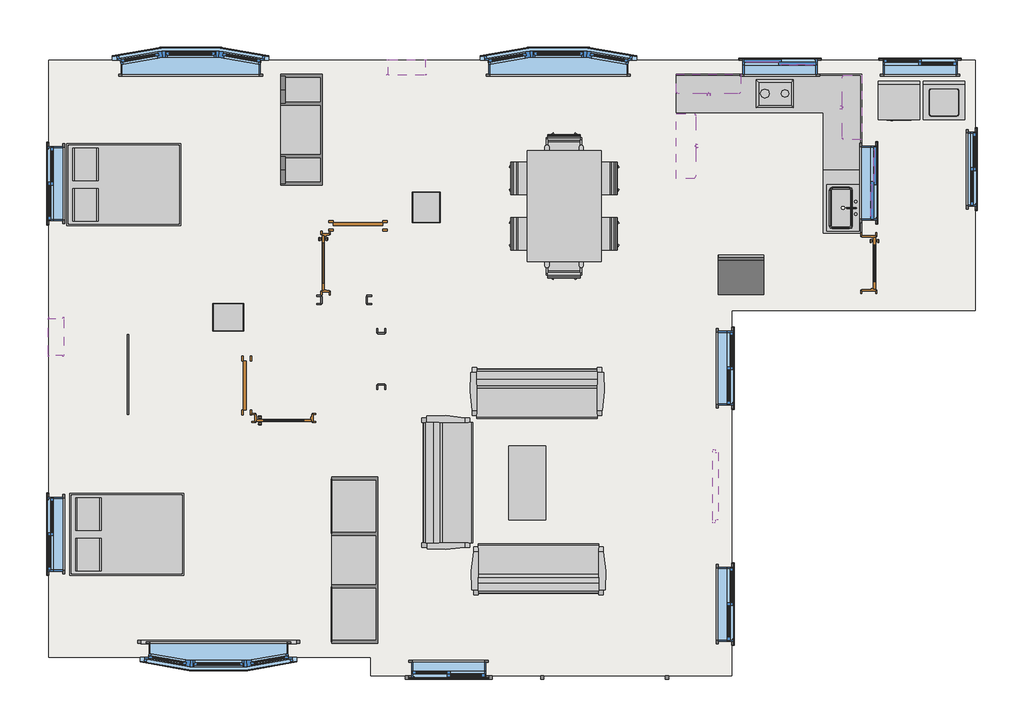
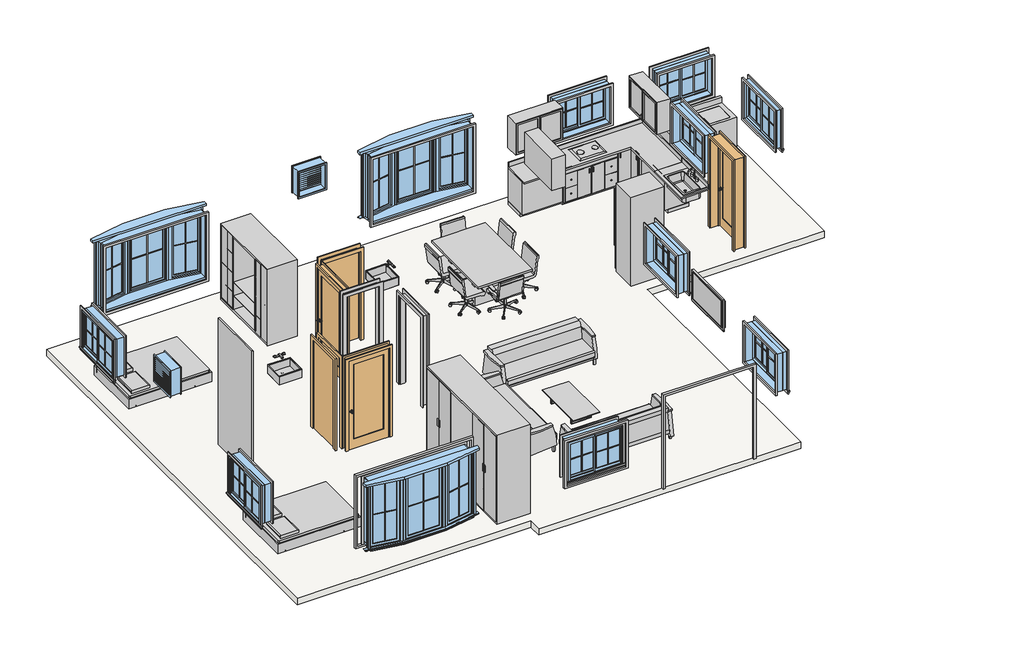
# One storey, incomplete: 54 proxies, 27 furniture elements, 14 windows, 5 doors, 3 flow terminals, 1 plate, 1 slab.
"""IFC4 building model written with IfcOpenShell, lengths in millimetres."""

from ifc_helpers import new_model, si_unit, frame, origin, place, context, project, spatial, polyline, outline, extrude, transform, mapped, element, save
from components import proxy_3c1fa1d0, proxy_97c73763, muntin_pattern_2x2_muntin_pattern_2x2_d8607f27, muntin_pattern_2x2_muntin_pattern_2x2_395d1e8c, muntin_pattern_2x2_muntin_pattern_2x2_0ac132d2, proxy_7d9a186d, proxy_dc468f74, proxy_76352e5b, trim_window_exterior_flat_with_sill_c4e67c73, trim_window_interior_flat_picture_frame_9ca7b173, trim_window_interior_flat_picture_frame_cf1733af, proxy_e75280ca, door_e2f2f551, door_a3feeac7, door_38851409, flow_terminal_cce4e9d2, flow_terminal_4d548711, furniture_e236c193, furniture_f415afdb, furniture_13b99e4d, furniture_b58f7881, casework_2_casework_2_327cef27, casework_3_casework_3_ac713c45, chair_task_chair_task_b7f3823b, chair_task_arms_chair_task_arms_fa5a08ef, furniture_738e865d, furniture_f6f93809, furniture_88072bd9, furniture_1f19b6cd, furniture_4a9d42a7, furniture_0c59c13b, furniture_0bcc43ae, furniture_5e39d705, furniture_92d3ea51, furniture_19fd8281, system_panel_glazed_349e9711, window_bf21e6cb, window_f2d8fef0, window_2eef0573, window_a4a981b4

model = new_model("IFC4")

# Units and contexts
model_context = context("Model", 3, world=origin())
ifc_project = project(units=[si_unit("LENGTHUNIT", "METRE", prefix="MILLI")], contexts=[model_context])

# Site, building, storey
site = spatial("IfcSite", under=ifc_project)
building = spatial("IfcBuilding", under=site)
storey = spatial("IfcBuildingStorey", under=building, Elevation=609.6)

# Proxies
placement = place(None, origin())
proxy_shape = proxy_3c1fa1d0(model_context)
element("IfcBuildingElementProxy", 1, Name="Cook Top-2 Unit : 12\" x 18\" 2", ObjectType="Cook Top-2 Unit : 12\" x 18\" 2", at=placement, inside=storey, context=model_context, shape_type="MappedRepresentation", body=[
    mapped(proxy_shape, transform((-6059.4169457, 11972.2965218, 609.6), x_axis=(0.0, 1.0, 0.0), y_axis=(-1.0, 0.0, 0.0), z_axis=(0.0, 0.0, 1.0))),
])
proxy_2_shape = proxy_97c73763(model_context)
element("IfcBuildingElementProxy", 2, Name="Dryer : 27\" x 25\" x 35\"", ObjectType="Dryer : 27\" x 25\" x 35\"", at=placement, inside=storey, context=model_context, shape_type="MappedRepresentation", body=[
    mapped(proxy_2_shape, transform((-4423.9291976, 11619.535518, 609.6), x_axis=(1.0, 0.0, 0.0), y_axis=(0.0, 1.0, 0.0), z_axis=(0.0, 0.0, 1.0))),
])
muntin_pattern_2x2_muntin_pattern_2x2_shape = muntin_pattern_2x2_muntin_pattern_2x2_d8607f27(model_context)
element("IfcBuildingElementProxy", 3, Name="Muntin Pattern_2x2 : Muntin Pattern_2x2", ObjectType="Muntin Pattern_2x2 : Muntin Pattern_2x2", at=placement, inside=storey, context=model_context, shape_type="MappedRepresentation", body=[
    mapped(muntin_pattern_2x2_muntin_pattern_2x2_shape, transform((-15243.1667413, 2653.6715218, 1339.85), x_axis=(-1.0, 0.0, 0.0), y_axis=(0.0, -1.0, 0.0), z_axis=(0.0, 0.0, 1.0))),
])
element("IfcBuildingElementProxy", 4, Name="Muntin Pattern_2x2 : Muntin Pattern_2x2", ObjectType="Muntin Pattern_2x2 : Muntin Pattern_2x2", at=placement, inside=storey, context=model_context, shape_type="MappedRepresentation", body=[
    mapped(muntin_pattern_2x2_muntin_pattern_2x2_shape, transform((-15700.3667413, 12705.7215218, 1339.85), x_axis=(1.0, 0.0, 0.0), y_axis=(0.0, 1.0, 0.0), z_axis=(0.0, 0.0, 1.0))),
])
element("IfcBuildingElementProxy", 5, Name="Muntin Pattern_2x2 : Muntin Pattern_2x2", ObjectType="Muntin Pattern_2x2 : Muntin Pattern_2x2", at=placement, inside=storey, context=model_context, shape_type="MappedRepresentation", body=[
    mapped(muntin_pattern_2x2_muntin_pattern_2x2_shape, transform((-9651.9917413, 12705.7215218, 1339.85), x_axis=(1.0, 0.0, 0.0), y_axis=(0.0, 1.0, 0.0), z_axis=(0.0, 0.0, 1.0))),
])
muntin_pattern_2x2_muntin_pattern_2x2_2_shape = muntin_pattern_2x2_muntin_pattern_2x2_395d1e8c(model_context)
element("IfcBuildingElementProxy", 6, Name="Muntin Pattern_2x2 : Muntin Pattern_2x2", ObjectType="Muntin Pattern_2x2 : Muntin Pattern_2x2", at=placement, inside=storey, context=model_context, shape_type="MappedRepresentation", body=[
    mapped(muntin_pattern_2x2_muntin_pattern_2x2_2_shape, transform((-14406.7973738, 2718.2624794, 1339.85), x_axis=(-0.9848077530122097, -0.17364817766692092, 0.0), y_axis=(0.17364817766692092, -0.9848077530122097, 0.0), z_axis=(0.0, 0.0, 1.0))),
])
element("IfcBuildingElementProxy", 7, Name="Muntin Pattern_2x2 : Muntin Pattern_2x2", ObjectType="Muntin Pattern_2x2 : Muntin Pattern_2x2", at=placement, inside=storey, context=model_context, shape_type="MappedRepresentation", body=[
    mapped(muntin_pattern_2x2_muntin_pattern_2x2_2_shape, transform((-16079.5361088, 2718.2624794, 1339.85), x_axis=(-0.9848077530122065, 0.17364817766693974, 0.0), y_axis=(-0.17364817766693974, -0.9848077530122065, 0.0), z_axis=(0.0, 0.0, 1.0))),
])
element("IfcBuildingElementProxy", 8, Name="Muntin Pattern_2x2 : Muntin Pattern_2x2", ObjectType="Muntin Pattern_2x2 : Muntin Pattern_2x2", at=placement, inside=storey, context=model_context, shape_type="MappedRepresentation", body=[
    mapped(muntin_pattern_2x2_muntin_pattern_2x2_2_shape, transform((-16536.7361088, 12641.1305642, 1339.85), x_axis=(0.9848077530122097, 0.17364817766692092, 0.0), y_axis=(-0.17364817766692092, 0.9848077530122097, 0.0), z_axis=(0.0, 0.0, 1.0))),
])
element("IfcBuildingElementProxy", 9, Name="Muntin Pattern_2x2 : Muntin Pattern_2x2", ObjectType="Muntin Pattern_2x2 : Muntin Pattern_2x2", at=placement, inside=storey, context=model_context, shape_type="MappedRepresentation", body=[
    mapped(muntin_pattern_2x2_muntin_pattern_2x2_2_shape, transform((-14863.9973738, 12641.1305642, 1339.85), x_axis=(0.9848077530122065, -0.17364817766693974, 0.0), y_axis=(0.17364817766693974, 0.9848077530122065, 0.0), z_axis=(0.0, 0.0, 1.0))),
])
element("IfcBuildingElementProxy", 10, Name="Muntin Pattern_2x2 : Muntin Pattern_2x2", ObjectType="Muntin Pattern_2x2 : Muntin Pattern_2x2", at=placement, inside=storey, context=model_context, shape_type="MappedRepresentation", body=[
    mapped(muntin_pattern_2x2_muntin_pattern_2x2_2_shape, transform((-10488.3611088, 12641.1305642, 1339.85), x_axis=(0.9848077530122097, 0.17364817766692092, 0.0), y_axis=(-0.17364817766692092, 0.9848077530122097, 0.0), z_axis=(0.0, 0.0, 1.0))),
])
element("IfcBuildingElementProxy", 11, Name="Muntin Pattern_2x2 : Muntin Pattern_2x2", ObjectType="Muntin Pattern_2x2 : Muntin Pattern_2x2", at=placement, inside=storey, context=model_context, shape_type="MappedRepresentation", body=[
    mapped(muntin_pattern_2x2_muntin_pattern_2x2_2_shape, transform((-8815.6223738, 12641.1305642, 1339.85), x_axis=(0.9848077530122065, -0.17364817766693974, 0.0), y_axis=(0.17364817766693974, 0.9848077530122065, 0.0), z_axis=(0.0, 0.0, 1.0))),
])
muntin_pattern_2x2_muntin_pattern_2x2_3_shape = muntin_pattern_2x2_muntin_pattern_2x2_0ac132d2(model_context)
element("IfcBuildingElementProxy", 12, Name="Muntin Pattern_2x2 : Muntin Pattern_2x2", ObjectType="Muntin Pattern_2x2 : Muntin Pattern_2x2", at=placement, inside=storey, context=model_context, shape_type="MappedRepresentation", body=[
    mapped(muntin_pattern_2x2_muntin_pattern_2x2_3_shape, transform((-5719.7542413, 12540.6215218, 1835.15), x_axis=(1.0, 0.0, 0.0), y_axis=(0.0, 1.0, 0.0), z_axis=(0.0, 0.0, 1.0))),
])
element("IfcBuildingElementProxy", 13, Name="Muntin Pattern_2x2 : Muntin Pattern_2x2", ObjectType="Muntin Pattern_2x2 : Muntin Pattern_2x2", at=placement, inside=storey, context=model_context, shape_type="MappedRepresentation", body=[
    mapped(muntin_pattern_2x2_muntin_pattern_2x2_3_shape, transform((-6288.0792413, 12585.0715218, 1835.15), x_axis=(1.0, 0.0, 0.0), y_axis=(0.0, 1.0, 0.0), z_axis=(0.0, 0.0, 1.0))),
])
element("IfcBuildingElementProxy", 14, Name="Muntin Pattern_2x2 : Muntin Pattern_2x2", ObjectType="Muntin Pattern_2x2 : Muntin Pattern_2x2", at=placement, inside=storey, context=model_context, shape_type="MappedRepresentation", body=[
    mapped(muntin_pattern_2x2_muntin_pattern_2x2_3_shape, transform((-4486.2667413, 10291.1340218, 1809.75), x_axis=(0.0, -1.0, 0.0), y_axis=(1.0, 0.0, 0.0), z_axis=(0.0, 0.0, 1.0))),
])
element("IfcBuildingElementProxy", 15, Name="Muntin Pattern_2x2 : Muntin Pattern_2x2", ObjectType="Muntin Pattern_2x2 : Muntin Pattern_2x2", at=placement, inside=storey, context=model_context, shape_type="MappedRepresentation", body=[
    mapped(muntin_pattern_2x2_muntin_pattern_2x2_3_shape, transform((-4441.8167413, 10859.4590218, 1809.75), x_axis=(0.0, -1.0, 0.0), y_axis=(1.0, 0.0, 0.0), z_axis=(0.0, 0.0, 1.0))),
])
element("IfcBuildingElementProxy", 16, Name="Muntin Pattern_2x2 : Muntin Pattern_2x2", ObjectType="Muntin Pattern_2x2 : Muntin Pattern_2x2", at=placement, inside=storey, context=model_context, shape_type="MappedRepresentation", body=[
    mapped(muntin_pattern_2x2_muntin_pattern_2x2_3_shape, transform((-6848.4667413, 7243.1340218, 1606.55), x_axis=(0.0, -1.0, 0.0), y_axis=(1.0, 0.0, 0.0), z_axis=(0.0, 0.0, 1.0))),
])
element("IfcBuildingElementProxy", 17, Name="Muntin Pattern_2x2 : Muntin Pattern_2x2", ObjectType="Muntin Pattern_2x2 : Muntin Pattern_2x2", at=placement, inside=storey, context=model_context, shape_type="MappedRepresentation", body=[
    mapped(muntin_pattern_2x2_muntin_pattern_2x2_3_shape, transform((-6804.0167413, 7811.4590218, 1606.55), x_axis=(0.0, -1.0, 0.0), y_axis=(1.0, 0.0, 0.0), z_axis=(0.0, 0.0, 1.0))),
])
element("IfcBuildingElementProxy", 18, Name="Muntin Pattern_2x2 : Muntin Pattern_2x2", ObjectType="Muntin Pattern_2x2 : Muntin Pattern_2x2", at=placement, inside=storey, context=model_context, shape_type="MappedRepresentation", body=[
    mapped(muntin_pattern_2x2_muntin_pattern_2x2_3_shape, transform((-6848.4667413, 3356.9340218, 1606.55), x_axis=(0.0, -1.0, 0.0), y_axis=(1.0, 0.0, 0.0), z_axis=(0.0, 0.0, 1.0))),
])
element("IfcBuildingElementProxy", 19, Name="Muntin Pattern_2x2 : Muntin Pattern_2x2", ObjectType="Muntin Pattern_2x2 : Muntin Pattern_2x2", at=placement, inside=storey, context=model_context, shape_type="MappedRepresentation", body=[
    mapped(muntin_pattern_2x2_muntin_pattern_2x2_3_shape, transform((-6804.0167413, 3925.2590218, 1606.55), x_axis=(0.0, -1.0, 0.0), y_axis=(1.0, 0.0, 0.0), z_axis=(0.0, 0.0, 1.0))),
])
element("IfcBuildingElementProxy", 20, Name="Muntin Pattern_2x2 : Muntin Pattern_2x2", ObjectType="Muntin Pattern_2x2 : Muntin Pattern_2x2", at=placement, inside=storey, context=model_context, shape_type="MappedRepresentation", body=[
    mapped(muntin_pattern_2x2_muntin_pattern_2x2_3_shape, transform((-11739.5542413, 2513.9715218, 1606.55), x_axis=(-1.0, 0.0, 0.0), y_axis=(0.0, -1.0, 0.0), z_axis=(0.0, 0.0, 1.0))),
])
element("IfcBuildingElementProxy", 21, Name="Muntin Pattern_2x2 : Muntin Pattern_2x2", ObjectType="Muntin Pattern_2x2 : Muntin Pattern_2x2", at=placement, inside=storey, context=model_context, shape_type="MappedRepresentation", body=[
    mapped(muntin_pattern_2x2_muntin_pattern_2x2_3_shape, transform((-11171.2292413, 2469.5215218, 1606.55), x_axis=(-1.0, 0.0, 0.0), y_axis=(0.0, -1.0, 0.0), z_axis=(0.0, 0.0, 1.0))),
])
element("IfcBuildingElementProxy", 22, Name="Muntin Pattern_2x2 : Muntin Pattern_2x2", ObjectType="Muntin Pattern_2x2 : Muntin Pattern_2x2", at=placement, inside=storey, context=model_context, shape_type="MappedRepresentation", body=[
    mapped(muntin_pattern_2x2_muntin_pattern_2x2_3_shape, transform((-17980.0167413, 5077.7840218, 1606.55), x_axis=(0.0, 1.0, 0.0), y_axis=(-1.0, 0.0, 0.0), z_axis=(0.0, 0.0, 1.0))),
])
element("IfcBuildingElementProxy", 23, Name="Muntin Pattern_2x2 : Muntin Pattern_2x2", ObjectType="Muntin Pattern_2x2 : Muntin Pattern_2x2", at=placement, inside=storey, context=model_context, shape_type="MappedRepresentation", body=[
    mapped(muntin_pattern_2x2_muntin_pattern_2x2_3_shape, transform((-18024.4667413, 4509.4590218, 1606.55), x_axis=(0.0, 1.0, 0.0), y_axis=(-1.0, 0.0, 0.0), z_axis=(0.0, 0.0, 1.0))),
])
element("IfcBuildingElementProxy", 24, Name="Muntin Pattern_2x2 : Muntin Pattern_2x2", ObjectType="Muntin Pattern_2x2 : Muntin Pattern_2x2", at=placement, inside=storey, context=model_context, shape_type="MappedRepresentation", body=[
    mapped(muntin_pattern_2x2_muntin_pattern_2x2_3_shape, transform((-17980.0167413, 10849.9340218, 1606.55), x_axis=(0.0, 1.0, 0.0), y_axis=(-1.0, 0.0, 0.0), z_axis=(0.0, 0.0, 1.0))),
])
element("IfcBuildingElementProxy", 25, Name="Muntin Pattern_2x2 : Muntin Pattern_2x2", ObjectType="Muntin Pattern_2x2 : Muntin Pattern_2x2", at=placement, inside=storey, context=model_context, shape_type="MappedRepresentation", body=[
    mapped(muntin_pattern_2x2_muntin_pattern_2x2_3_shape, transform((-18024.4667413, 10281.6090218, 1606.55), x_axis=(0.0, 1.0, 0.0), y_axis=(-1.0, 0.0, 0.0), z_axis=(0.0, 0.0, 1.0))),
])
element("IfcBuildingElementProxy", 26, Name="Muntin Pattern_2x2 : Muntin Pattern_2x2", ObjectType="Muntin Pattern_2x2 : Muntin Pattern_2x2", at=placement, inside=storey, context=model_context, shape_type="MappedRepresentation", body=[
    mapped(muntin_pattern_2x2_muntin_pattern_2x2_3_shape, transform((-2847.9667413, 10519.7340218, 1657.35), x_axis=(0.0, -1.0, 0.0), y_axis=(1.0, 0.0, 0.0), z_axis=(0.0, 0.0, 1.0))),
])
element("IfcBuildingElementProxy", 27, Name="Muntin Pattern_2x2 : Muntin Pattern_2x2", ObjectType="Muntin Pattern_2x2 : Muntin Pattern_2x2", at=placement, inside=storey, context=model_context, shape_type="MappedRepresentation", body=[
    mapped(muntin_pattern_2x2_muntin_pattern_2x2_3_shape, transform((-2803.5167413, 11088.0590218, 1657.35), x_axis=(0.0, -1.0, 0.0), y_axis=(1.0, 0.0, 0.0), z_axis=(0.0, 0.0, 1.0))),
])
element("IfcBuildingElementProxy", 28, Name="Muntin Pattern_2x2 : Muntin Pattern_2x2", ObjectType="Muntin Pattern_2x2 : Muntin Pattern_2x2", at=placement, inside=storey, context=model_context, shape_type="MappedRepresentation", body=[
    mapped(muntin_pattern_2x2_muntin_pattern_2x2_3_shape, transform((-3414.7042413, 12540.6215218, 1708.15), x_axis=(1.0, 0.0, 0.0), y_axis=(0.0, 1.0, 0.0), z_axis=(0.0, 0.0, 1.0))),
])
element("IfcBuildingElementProxy", 29, Name="Muntin Pattern_2x2 : Muntin Pattern_2x2", ObjectType="Muntin Pattern_2x2 : Muntin Pattern_2x2", at=placement, inside=storey, context=model_context, shape_type="MappedRepresentation", body=[
    mapped(muntin_pattern_2x2_muntin_pattern_2x2_3_shape, transform((-3983.0292413, 12585.0715218, 1708.15), x_axis=(1.0, 0.0, 0.0), y_axis=(0.0, 1.0, 0.0), z_axis=(0.0, 0.0, 1.0))),
])
proxy_3_shape = proxy_7d9a186d(model_context)
element("IfcBuildingElementProxy", 30, Name="Passage Opening-Cased : 30\" x 84\"", ObjectType="Passage Opening-Cased : 30\" x 84\"", at=placement, inside=storey, context=model_context, shape_type="MappedRepresentation", body=[
    mapped(proxy_3_shape, transform((-13184.430398, 8651.2465218, 609.6), x_axis=(-1.0, 0.0, 0.0), y_axis=(0.0, -1.0, 0.0), z_axis=(0.0, 0.0, 1.0))),
])
proxy_4_shape = proxy_dc468f74(model_context)
element("IfcBuildingElementProxy", 31, Name="Passage Opening-Cased : 34\" x 84\"", ObjectType="Passage Opening-Cased : 34\" x 84\"", at=placement, inside=storey, context=model_context, shape_type="MappedRepresentation", body=[
    mapped(proxy_4_shape, transform((-12566.6417413, 7687.8851785, 609.6), x_axis=(0.0, 1.0, 0.0), y_axis=(-1.0, 0.0, 0.0), z_axis=(0.0, 0.0, 1.0))),
])
proxy_5_shape = proxy_76352e5b(model_context)
element("IfcBuildingElementProxy", 32, Name="Refrigerator-Built-in : 30\" x 24\" LH", ObjectType="Refrigerator-Built-in : 30\" x 24\" LH", at=placement, inside=storey, context=model_context, shape_type="MappedRepresentation", body=[
    mapped(proxy_5_shape, transform((-6648.4417413, 9027.8725503, 609.6), x_axis=(1.0, 0.0, 0.0), y_axis=(0.0, 1.0, 0.0), z_axis=(0.0, 0.0, 1.0))),
])
trim_window_exterior_flat_with_sill_shape = trim_window_exterior_flat_with_sill_c4e67c73(model_context)
element("IfcBuildingElementProxy", 33, Name="Trim-Window-Exterior-Flat : with Sill", ObjectType="Trim-Window-Exterior-Flat : with Sill", at=placement, inside=storey, context=model_context, shape_type="MappedRepresentation", body=[
    mapped(trim_window_exterior_flat_with_sill_shape, transform((-6003.9167413, 12594.5965218, 2667.0), x_axis=(-1.0, 0.0, 0.0), y_axis=(0.0, 0.0, 1.0), z_axis=(0.0, 1.0, 0.0))),
])
element("IfcBuildingElementProxy", 34, Name="Trim-Window-Exterior-Flat : with Sill", ObjectType="Trim-Window-Exterior-Flat : with Sill", at=placement, inside=storey, context=model_context, shape_type="MappedRepresentation", body=[
    mapped(trim_window_exterior_flat_with_sill_shape, transform((-4432.2917413, 10575.2965218, 2641.6), x_axis=(0.0, 1.0, 0.0), y_axis=(0.0, 0.0, 1.0), z_axis=(1.0, 0.0, 0.0))),
])
element("IfcBuildingElementProxy", 35, Name="Trim-Window-Exterior-Flat : with Sill", ObjectType="Trim-Window-Exterior-Flat : with Sill", at=placement, inside=storey, context=model_context, shape_type="MappedRepresentation", body=[
    mapped(trim_window_exterior_flat_with_sill_shape, transform((-6794.4917413, 7527.2965218, 2438.4), x_axis=(0.0, 1.0, 0.0), y_axis=(0.0, 0.0, 1.0), z_axis=(1.0, 0.0, 0.0))),
])
element("IfcBuildingElementProxy", 36, Name="Trim-Window-Exterior-Flat : with Sill", ObjectType="Trim-Window-Exterior-Flat : with Sill", at=placement, inside=storey, context=model_context, shape_type="MappedRepresentation", body=[
    mapped(trim_window_exterior_flat_with_sill_shape, transform((-6794.4917413, 3641.0965218, 2438.4), x_axis=(0.0, 1.0, 0.0), y_axis=(0.0, 0.0, 1.0), z_axis=(1.0, 0.0, 0.0))),
])
element("IfcBuildingElementProxy", 37, Name="Trim-Window-Exterior-Flat : with Sill", ObjectType="Trim-Window-Exterior-Flat : with Sill", at=placement, inside=storey, context=model_context, shape_type="MappedRepresentation", body=[
    mapped(trim_window_exterior_flat_with_sill_shape, transform((-11455.3917413, 2459.9965218, 2438.4), x_axis=(1.0, 0.0, 0.0), y_axis=(0.0, 0.0, 1.0), z_axis=(0.0, -1.0, 0.0))),
])
element("IfcBuildingElementProxy", 38, Name="Trim-Window-Exterior-Flat : with Sill", ObjectType="Trim-Window-Exterior-Flat : with Sill", at=placement, inside=storey, context=model_context, shape_type="MappedRepresentation", body=[
    mapped(trim_window_exterior_flat_with_sill_shape, transform((-18033.9917413, 4793.6215218, 2438.4), x_axis=(0.0, -1.0, 0.0), y_axis=(0.0, 0.0, 1.0), z_axis=(-1.0, 0.0, 0.0))),
])
element("IfcBuildingElementProxy", 39, Name="Trim-Window-Exterior-Flat : with Sill", ObjectType="Trim-Window-Exterior-Flat : with Sill", at=placement, inside=storey, context=model_context, shape_type="MappedRepresentation", body=[
    mapped(trim_window_exterior_flat_with_sill_shape, transform((-18033.9917413, 10565.7715218, 2438.4), x_axis=(0.0, -1.0, 0.0), y_axis=(0.0, 0.0, 1.0), z_axis=(-1.0, 0.0, 0.0))),
])
element("IfcBuildingElementProxy", 40, Name="Trim-Window-Exterior-Flat : with Sill", ObjectType="Trim-Window-Exterior-Flat : with Sill", at=placement, inside=storey, context=model_context, shape_type="MappedRepresentation", body=[
    mapped(trim_window_exterior_flat_with_sill_shape, transform((-2793.9917413, 10803.8965218, 2489.2), x_axis=(0.0, 1.0, 0.0), y_axis=(0.0, 0.0, 1.0), z_axis=(1.0, 0.0, 0.0))),
])
element("IfcBuildingElementProxy", 41, Name="Trim-Window-Exterior-Flat : with Sill", ObjectType="Trim-Window-Exterior-Flat : with Sill", at=placement, inside=storey, context=model_context, shape_type="MappedRepresentation", body=[
    mapped(trim_window_exterior_flat_with_sill_shape, transform((-3698.8667413, 12594.5965218, 2540.0), x_axis=(-1.0, 0.0, 0.0), y_axis=(0.0, 0.0, 1.0), z_axis=(0.0, 1.0, 0.0))),
])
trim_window_interior_flat_picture_frame_shape = trim_window_interior_flat_picture_frame_9ca7b173(model_context)
element("IfcBuildingElementProxy", 42, Name="Trim-Window-Interior-Flat : Picture Frame", ObjectType="Trim-Window-Interior-Flat : Picture Frame", at=placement, inside=storey, context=model_context, shape_type="MappedRepresentation", body=[
    mapped(trim_window_interior_flat_picture_frame_shape, transform((-15243.1667413, 2993.3965218, 2794.0), x_axis=(-1.0, 0.0, 0.0), y_axis=(0.0, 0.0, 1.0), z_axis=(0.0, 1.0, 0.0))),
])
element("IfcBuildingElementProxy", 43, Name="Trim-Window-Interior-Flat : Picture Frame", ObjectType="Trim-Window-Interior-Flat : Picture Frame", at=placement, inside=storey, context=model_context, shape_type="MappedRepresentation", body=[
    mapped(trim_window_interior_flat_picture_frame_shape, transform((-15700.3667413, 12365.9965218, 2794.0), x_axis=(1.0, 0.0, 0.0), y_axis=(0.0, 0.0, 1.0), z_axis=(0.0, -1.0, 0.0))),
])
element("IfcBuildingElementProxy", 44, Name="Trim-Window-Interior-Flat : Picture Frame", ObjectType="Trim-Window-Interior-Flat : Picture Frame", at=placement, inside=storey, context=model_context, shape_type="MappedRepresentation", body=[
    mapped(trim_window_interior_flat_picture_frame_shape, transform((-9651.9917413, 12365.9965218, 2794.0), x_axis=(1.0, 0.0, 0.0), y_axis=(0.0, 0.0, 1.0), z_axis=(0.0, -1.0, 0.0))),
])
trim_window_interior_flat_picture_frame_2_shape = trim_window_interior_flat_picture_frame_cf1733af(model_context)
element("IfcBuildingElementProxy", 45, Name="Trim-Window-Interior-Flat : Picture Frame", ObjectType="Trim-Window-Interior-Flat : Picture Frame", at=placement, inside=storey, context=model_context, shape_type="MappedRepresentation", body=[
    mapped(trim_window_interior_flat_picture_frame_2_shape, transform((-6003.9167413, 12365.9965218, 2667.0), x_axis=(1.0, 0.0, 0.0), y_axis=(0.0, 0.0, 1.0), z_axis=(0.0, -1.0, 0.0))),
])
element("IfcBuildingElementProxy", 46, Name="Trim-Window-Interior-Flat : Picture Frame", ObjectType="Trim-Window-Interior-Flat : Picture Frame", at=placement, inside=storey, context=model_context, shape_type="MappedRepresentation", body=[
    mapped(trim_window_interior_flat_picture_frame_2_shape, transform((-4660.8917413, 10575.2965218, 2641.6), x_axis=(0.0, -1.0, 0.0), y_axis=(0.0, 0.0, 1.0), z_axis=(-1.0, 0.0, 0.0))),
])
element("IfcBuildingElementProxy", 47, Name="Trim-Window-Interior-Flat : Picture Frame", ObjectType="Trim-Window-Interior-Flat : Picture Frame", at=placement, inside=storey, context=model_context, shape_type="MappedRepresentation", body=[
    mapped(trim_window_interior_flat_picture_frame_2_shape, transform((-7023.0917413, 7527.2965218, 2438.4), x_axis=(0.0, -1.0, 0.0), y_axis=(0.0, 0.0, 1.0), z_axis=(-1.0, 0.0, 0.0))),
])
element("IfcBuildingElementProxy", 48, Name="Trim-Window-Interior-Flat : Picture Frame", ObjectType="Trim-Window-Interior-Flat : Picture Frame", at=placement, inside=storey, context=model_context, shape_type="MappedRepresentation", body=[
    mapped(trim_window_interior_flat_picture_frame_2_shape, transform((-7023.0917413, 3641.0965218, 2438.4), x_axis=(0.0, -1.0, 0.0), y_axis=(0.0, 0.0, 1.0), z_axis=(-1.0, 0.0, 0.0))),
])
element("IfcBuildingElementProxy", 49, Name="Trim-Window-Interior-Flat : Picture Frame", ObjectType="Trim-Window-Interior-Flat : Picture Frame", at=placement, inside=storey, context=model_context, shape_type="MappedRepresentation", body=[
    mapped(trim_window_interior_flat_picture_frame_2_shape, transform((-11455.3917413, 2688.5965218, 2438.4), x_axis=(-1.0, 0.0, 0.0), y_axis=(0.0, 0.0, 1.0), z_axis=(0.0, 1.0, 0.0))),
])
element("IfcBuildingElementProxy", 50, Name="Trim-Window-Interior-Flat : Picture Frame", ObjectType="Trim-Window-Interior-Flat : Picture Frame", at=placement, inside=storey, context=model_context, shape_type="MappedRepresentation", body=[
    mapped(trim_window_interior_flat_picture_frame_2_shape, transform((-17805.3917413, 4793.6215218, 2438.4), x_axis=(0.0, 1.0, 0.0), y_axis=(0.0, 0.0, 1.0), z_axis=(1.0, 0.0, 0.0))),
])
element("IfcBuildingElementProxy", 51, Name="Trim-Window-Interior-Flat : Picture Frame", ObjectType="Trim-Window-Interior-Flat : Picture Frame", at=placement, inside=storey, context=model_context, shape_type="MappedRepresentation", body=[
    mapped(trim_window_interior_flat_picture_frame_2_shape, transform((-17805.3917413, 10565.7715218, 2438.4), x_axis=(0.0, 1.0, 0.0), y_axis=(0.0, 0.0, 1.0), z_axis=(1.0, 0.0, 0.0))),
])
element("IfcBuildingElementProxy", 52, Name="Trim-Window-Interior-Flat : Picture Frame", ObjectType="Trim-Window-Interior-Flat : Picture Frame", at=placement, inside=storey, context=model_context, shape_type="MappedRepresentation", body=[
    mapped(trim_window_interior_flat_picture_frame_2_shape, transform((-2908.2917413, 10803.8965218, 2489.2), x_axis=(0.0, -1.0, 0.0), y_axis=(0.0, 0.0, 1.0), z_axis=(-1.0, 0.0, 0.0))),
])
element("IfcBuildingElementProxy", 53, Name="Trim-Window-Interior-Flat : Picture Frame", ObjectType="Trim-Window-Interior-Flat : Picture Frame", at=placement, inside=storey, context=model_context, shape_type="MappedRepresentation", body=[
    mapped(trim_window_interior_flat_picture_frame_2_shape, transform((-3698.8667413, 12365.9965218, 2540.0), x_axis=(1.0, 0.0, 0.0), y_axis=(0.0, 0.0, 1.0), z_axis=(0.0, -1.0, 0.0))),
])
proxy_6_shape = proxy_e75280ca(model_context)
element("IfcBuildingElementProxy", 54, Name="Washer : 27\" x 25\" x 35\"", ObjectType="Washer : 27\" x 25\" x 35\"", at=placement, inside=storey, context=model_context, shape_type="MappedRepresentation", body=[
    mapped(proxy_6_shape, transform((-3728.7592098, 11655.046957, 609.6), x_axis=(1.0, 0.0, 0.0), y_axis=(0.0, 1.0, 0.0), z_axis=(0.0, 0.0, 1.0))),
])

# Doors
door_shape = door_e2f2f551(model_context)
element("IfcDoor", 55, ObjectType="Door-Interior-Single-1_Panel-Wood : 34\" x 84\"", at=placement, inside=storey, context=model_context, shape_type="MappedRepresentation", body=[
    mapped(door_shape, transform((-4543.4167413, 9254.4965218, 609.6), x_axis=(0.0, -1.0, 0.0), y_axis=(1.0, 0.0, 0.0), z_axis=(0.0, 0.0, 1.0))),
])
door_2_shape = door_a3feeac7(model_context)
element("IfcDoor", 56, ObjectType="Door-Interior-Single-1_Panel-Wood : 36\" x 84\"", at=placement, inside=storey, context=model_context, shape_type="MappedRepresentation", body=[
    mapped(door_2_shape, transform((-14166.8417413, 6704.9715218, 609.6), x_axis=(1.0, 0.0, 0.0), y_axis=(0.0, 1.0, 0.0), z_axis=(0.0, 0.0, 1.0))),
])
element("IfcDoor", 57, ObjectType="Door-Interior-Single-1_Panel-Wood : 36\" x 84\"", at=placement, inside=storey, context=model_context, shape_type="MappedRepresentation", body=[
    mapped(door_2_shape, transform((-13484.2167413, 9260.8465218, 609.6), x_axis=(0.0, -1.0, 0.0), y_axis=(1.0, 0.0, 0.0), z_axis=(0.0, 0.0, 1.0))),
])
door_3_shape = door_38851409(model_context)
element("IfcDoor", 58, ObjectType="Single-Flush : 32\" x 84\"", at=placement, inside=storey, context=model_context, shape_type="MappedRepresentation", body=[
    mapped(door_3_shape, transform((-12947.6417413, 9870.4465218, 609.6), x_axis=(-1.0, 0.0, 0.0), y_axis=(0.0, -1.0, 0.0), z_axis=(0.0, 0.0, 1.0))),
])
element("IfcDoor", 59, ObjectType="Single-Flush : 32\" x 84\"", at=placement, inside=storey, context=model_context, shape_type="MappedRepresentation", body=[
    mapped(door_3_shape, transform((-14776.4417413, 7241.5465218, 609.6), x_axis=(0.0, -1.0, 0.0), y_axis=(1.0, 0.0, 0.0), z_axis=(0.0, 0.0, 1.0))),
])

# Flow terminals
flow_terminal_shape = flow_terminal_cce4e9d2(model_context)
element("IfcFlowTerminal", 60, ObjectType="Sink - Work : 20\"x18\"", at=placement, inside=storey, context=model_context, shape_type="MappedRepresentation", body=[
    mapped(flow_terminal_shape, transform((-11595.0917413, 10175.2465218, 1524.0), x_axis=(0.0, -1.0, 0.0), y_axis=(1.0, 0.0, 0.0), z_axis=(0.0, 0.0, 1.0))),
])
element("IfcFlowTerminal", 61, ObjectType="Sink - Work : 20\"x18\"", at=placement, inside=storey, context=model_context, shape_type="MappedRepresentation", body=[
    mapped(flow_terminal_shape, transform((-15081.2417413, 8594.0965218, 1524.0), x_axis=(1.0, 0.0, 0.0), y_axis=(0.0, 1.0, 0.0), z_axis=(0.0, 0.0, 1.0))),
])
flow_terminal_2_shape = flow_terminal_4d548711(model_context)
element("IfcFlowTerminal", 62, ObjectType="Sink Kitchen-Single : 30\" x 21\"", at=placement, inside=storey, context=model_context, shape_type="MappedRepresentation", body=[
    mapped(flow_terminal_2_shape, transform((-4968.0371424, 10181.4107624, 609.6), x_axis=(0.0, -1.0, 0.0), y_axis=(1.0, 0.0, 0.0), z_axis=(0.0, 0.0, 1.0))),
])

# Furniture
furniture_shape = furniture_e236c193(model_context)
element("IfcFurniture", 63, ObjectType="48\" 2", at=placement, inside=storey, context=model_context, shape_type="MappedRepresentation", body=[
    mapped(furniture_shape, transform((-6275.7367013, 12365.9965218, 609.6), x_axis=(1.0, 0.0, 0.0), y_axis=(0.0, 1.0, 0.0), z_axis=(0.0, 0.0, 1.0))),
])
furniture_2_shape = furniture_f415afdb(model_context)
element("IfcFurniture", 64, ObjectType="Base Cabinet-Combo01 : 30\" 2", at=placement, inside=storey, context=model_context, shape_type="MappedRepresentation", body=[
    mapped(furniture_2_shape, transform((-7270.4294462, 12365.9965218, 609.6), x_axis=(1.0, 0.0, 0.0), y_axis=(0.0, 1.0, 0.0), z_axis=(0.0, 0.0, 1.0))),
])
element("IfcFurniture", 65, ObjectType="Base Cabinet-Combo01 : 30\" 2", at=placement, inside=storey, context=model_context, shape_type="MappedRepresentation", body=[
    mapped(furniture_2_shape, transform((-4660.8917413, 11026.4588169, 609.6), x_axis=(0.0, -1.0, 0.0), y_axis=(1.0, 0.0, 0.0), z_axis=(0.0, 0.0, 1.0))),
])
furniture_3_shape = furniture_13b99e4d(model_context)
element("IfcFurniture", 66, ObjectType="Base Cabinet-Corner Unit-Square : 36\" 2", at=placement, inside=storey, context=model_context, shape_type="MappedRepresentation", body=[
    mapped(furniture_3_shape, transform((-5187.6294462, 12365.9965218, 609.6), x_axis=(1.0, 0.0, 0.0), y_axis=(0.0, 1.0, 0.0), z_axis=(0.0, 0.0, 1.0))),
])
furniture_4_shape = furniture_b58f7881(model_context)
element("IfcFurniture", 67, ObjectType="Bed-Box : Double 53\" x 74\"", at=placement, inside=storey, context=model_context, shape_type="MappedRepresentation", body=[
    mapped(furniture_4_shape, transform((-17036.5212495, 10210.7440628, 609.6), x_axis=(0.0, 1.0, 0.0), y_axis=(-1.0, 0.0, 0.0), z_axis=(0.0, 0.0, 1.0))),
])
element("IfcFurniture", 68, ObjectType="Bed-Box : Double 53\" x 74\"", at=placement, inside=storey, context=model_context, shape_type="MappedRepresentation", body=[
    mapped(furniture_4_shape, transform((-16985.7212495, 4451.2940628, 609.6), x_axis=(0.0, 1.0, 0.0), y_axis=(-1.0, 0.0, 0.0), z_axis=(0.0, 0.0, 1.0))),
])
casework_2_casework_2_shape = casework_2_casework_2_327cef27(model_context)
element("IfcFurniture", 69, ObjectType="Casework 2 : Casework 2", at=placement, inside=storey, context=model_context, shape_type="MappedRepresentation", body=[
    mapped(casework_2_casework_2_shape, transform((0.0, 0.0, 0.0), x_axis=(1.0, 0.0, 0.0), y_axis=(0.0, 1.0, 0.0), z_axis=(0.0, 0.0, 1.0))),
])
casework_3_casework_3_shape = casework_3_casework_3_ac713c45(model_context)
element("IfcFurniture", 70, ObjectType="Casework 3 : Casework 3", at=placement, inside=storey, context=model_context, shape_type="MappedRepresentation", body=[
    mapped(casework_3_casework_3_shape, transform((0.0, 0.0, 0.0), x_axis=(1.0, 0.0, 0.0), y_axis=(0.0, 1.0, 0.0), z_axis=(0.0, 0.0, 1.0))),
])
chair_task_chair_task_shape = chair_task_chair_task_b7f3823b(model_context)
element("IfcFurniture", 71, ObjectType="Chair-Task : Chair-Task", at=placement, inside=storey, context=model_context, shape_type="MappedRepresentation", body=[
    mapped(chair_task_chair_task_shape, transform((-10185.2876429, 10792.4873415, 609.6), x_axis=(0.0, -1.0, 0.0), y_axis=(1.0, 0.0, 0.0), z_axis=(0.0, 0.0, 1.0))),
])
element("IfcFurniture", 72, ObjectType="Chair-Task : Chair-Task", at=placement, inside=storey, context=model_context, shape_type="MappedRepresentation", body=[
    mapped(chair_task_chair_task_shape, transform((-8928.1958397, 10510.5057021, 609.6), x_axis=(0.0, 1.0, 0.0), y_axis=(-1.0, 0.0, 0.0), z_axis=(0.0, 0.0, 1.0))),
])
element("IfcFurniture", 73, ObjectType="Chair-Task : Chair-Task", at=placement, inside=storey, context=model_context, shape_type="MappedRepresentation", body=[
    mapped(chair_task_chair_task_shape, transform((-10185.2876429, 9878.0873415, 609.6), x_axis=(0.0, -1.0, 0.0), y_axis=(1.0, 0.0, 0.0), z_axis=(0.0, 0.0, 1.0))),
])
element("IfcFurniture", 74, ObjectType="Chair-Task : Chair-Task", at=placement, inside=storey, context=model_context, shape_type="MappedRepresentation", body=[
    mapped(chair_task_chair_task_shape, transform((-8928.1958397, 9596.1057021, 609.6), x_axis=(0.0, 1.0, 0.0), y_axis=(-1.0, 0.0, 0.0), z_axis=(0.0, 0.0, 1.0))),
])
chair_task_arms_chair_task_arms_shape = chair_task_arms_chair_task_arms_fa5a08ef(model_context)
element("IfcFurniture", 75, ObjectType="Chair-Task Arms : Chair-Task Arms", at=placement, inside=storey, context=model_context, shape_type="MappedRepresentation", body=[
    mapped(chair_task_arms_chair_task_arms_shape, transform((-9697.732561, 9260.9506202, 609.6), x_axis=(1.0, 0.0, 0.0), y_axis=(0.0, 1.0, 0.0), z_axis=(0.0, 0.0, 1.0))),
])
element("IfcFurniture", 76, ObjectType="Chair-Task Arms : Chair-Task Arms", at=placement, inside=storey, context=model_context, shape_type="MappedRepresentation", body=[
    mapped(chair_task_arms_chair_task_arms_shape, transform((-9415.7509216, 11127.6424234, 609.6), x_axis=(-1.0, 0.0, 0.0), y_axis=(0.0, -1.0, 0.0), z_axis=(0.0, 0.0, 1.0))),
])
furniture_5_shape = furniture_738e865d(model_context)
element("IfcFurniture", 77, ObjectType="Counter Top w Sink Hole : 24\" Depth", at=placement, inside=storey, context=model_context, shape_type="MappedRepresentation", body=[
    mapped(furniture_5_shape, transform((-4660.8917413, 9590.7342267, 609.6), x_axis=(0.0, -1.0, 0.0), y_axis=(1.0, 0.0, 0.0), z_axis=(0.0, 0.0, 1.0))),
])
furniture_6_shape = furniture_f6f93809(model_context)
element("IfcFurniture", 78, ObjectType="Counter Top-L Shaped : 24\" Depth", at=placement, inside=storey, context=model_context, shape_type="MappedRepresentation", body=[
    mapped(furniture_6_shape, transform((-4660.8917413, 11165.5342267, 609.6), x_axis=(0.0, -1.0, 0.0), y_axis=(1.0, 0.0, 0.0), z_axis=(0.0, 0.0, 1.0))),
])
furniture_7_shape = furniture_88072bd9(model_context)
element("IfcFurniture", 79, ObjectType="Entertainment Center.0001 : 72\" x 72\" x 24\"", at=placement, inside=storey, context=model_context, shape_type="MappedRepresentation", body=[
    mapped(furniture_7_shape, transform((-13436.5917413, 11451.5965218, 609.6), x_axis=(0.0, -1.0, 0.0), y_axis=(1.0, 0.0, 0.0), z_axis=(0.0, 0.0, 1.0))),
])
furniture_8_shape = furniture_1f19b6cd(model_context)
element("IfcFurniture", 80, ObjectType="Entertainment Center.0001 : 96\" x 84\" x 30\"", at=placement, inside=storey, context=model_context, shape_type="MappedRepresentation", body=[
    mapped(furniture_8_shape, transform((-12598.3917413, 4364.9965218, 609.6), x_axis=(0.0, -1.0, 0.0), y_axis=(1.0, 0.0, 0.0), z_axis=(0.0, 0.0, 1.0))),
])
furniture_9_shape = furniture_4a9d42a7(model_context)
element("IfcFurniture", 81, ObjectType="Sofa-Pensi : 84\"", at=placement, inside=storey, context=model_context, shape_type="MappedRepresentation", body=[
    mapped(furniture_9_shape, transform((-11203.6819052, 5362.7402718, 609.6), x_axis=(0.0, 1.0, 0.0), y_axis=(-1.0, 0.0, 0.0), z_axis=(0.0, 0.0, 1.0))),
])
element("IfcFurniture", 82, ObjectType="Sofa-Pensi : 84\"", at=placement, inside=storey, context=model_context, shape_type="MappedRepresentation", body=[
    mapped(furniture_9_shape, transform((-10279.8479913, 6843.7866857, 609.6), x_axis=(1.0, 0.0, 0.0), y_axis=(0.0, 1.0, 0.0), z_axis=(0.0, 0.0, 1.0))),
])
element("IfcFurniture", 83, ObjectType="Sofa-Pensi : 84\"", at=placement, inside=storey, context=model_context, shape_type="MappedRepresentation", body=[
    mapped(furniture_9_shape, transform((-9697.2354913, 4489.7063579, 609.6), x_axis=(-1.0, 0.0, 0.0), y_axis=(0.0, -1.0, 0.0), z_axis=(0.0, 0.0, 1.0))),
])
furniture_10_shape = furniture_0c59c13b(model_context)
element("IfcFurniture", 84, ObjectType="Table-Coffee Rectangular : 48\" x 24\"", at=placement, inside=storey, context=model_context, shape_type="MappedRepresentation", body=[
    mapped(furniture_10_shape, transform((-9796.7309095, 5028.0128915, 609.6), x_axis=(0.0, 1.0, 0.0), y_axis=(-1.0, 0.0, 0.0), z_axis=(0.0, 0.0, 1.0))),
])
furniture_11_shape = furniture_0bcc43ae(model_context)
element("IfcFurniture", 85, ObjectType="Table-Conference2 w Chairs : 48\" x 144\" 2", at=placement, inside=storey, context=model_context, shape_type="MappedRepresentation", body=[
    mapped(furniture_11_shape, transform((-9556.7417413, 10194.2965218, 609.6), x_axis=(0.0, 1.0, 0.0), y_axis=(-1.0, 0.0, 0.0), z_axis=(0.0, 0.0, 1.0))),
])
furniture_12_shape = furniture_5e39d705(model_context)
element("IfcFurniture", 86, ObjectType="Television-Plasma : 50\"", at=placement, inside=storey, context=model_context, shape_type="MappedRepresentation", body=[
    mapped(furniture_12_shape, transform((-7023.0917413, 5641.3465218, 1828.8), x_axis=(0.0, -1.0, 0.0), y_axis=(1.0, 0.0, 0.0), z_axis=(0.0, 0.0, 1.0))),
])
furniture_13_shape = furniture_92d3ea51(model_context)
element("IfcFurniture", 87, ObjectType="Upper Cabinet-Double Door w Glass-Wall : 42\"", at=placement, inside=storey, context=model_context, shape_type="MappedRepresentation", body=[
    mapped(furniture_13_shape, transform((-7766.0417413, 11214.6676846, 609.6), x_axis=(0.0, -1.0, 0.0), y_axis=(1.0, 0.0, 0.0), z_axis=(0.0, 0.0, 1.0))),
])
furniture_14_shape = furniture_19fd8281(model_context)
element("IfcFurniture", 88, ObjectType="Upper Cabinet-Double Door w Glass-Wall : 42\"", at=placement, inside=storey, context=model_context, shape_type="MappedRepresentation", body=[
    mapped(furniture_14_shape, transform((-4546.5917413, 11790.125359, 609.6), x_axis=(0.0, 1.0, 0.0), y_axis=(-1.0, 0.0, 0.0), z_axis=(0.0, 0.0, 1.0))),
])
element("IfcFurniture", 89, ObjectType="Upper Cabinet-Double Door w Glass-Wall : 42\"", at=placement, inside=storey, context=model_context, shape_type="MappedRepresentation", body=[
    mapped(furniture_14_shape, transform((-7152.0705785, 12480.2965218, 609.6), x_axis=(-1.0, 0.0, 0.0), y_axis=(0.0, -1.0, 0.0), z_axis=(0.0, 0.0, 1.0))),
])

# Plate
system_panel_glazed_shape = system_panel_glazed_349e9711(model_context)
element("IfcPlate", 90, ObjectType="System Panel : Glazed", at=placement, inside=storey, context=model_context, shape_type="MappedRepresentation", body=[
    mapped(system_panel_glazed_shape, transform((-16700.4917413, 7422.5215218, 609.6), x_axis=(0.0, 1.0, 0.0), y_axis=(-1.0, 0.0, 0.0), z_axis=(0.0, 0.0, 1.0))),
])

# Slab
element("IfcSlab", 91, ObjectType="Generic - 6\"", at=placement, inside=storey, context=model_context, shape_type="SweptSolid", body=[
    extrude(outline(polyline([(-2793.9917413, 12594.5965218), (-2793.9917413, 8479.7965218), (-6794.4917413, 8479.7965218), (-6794.4917413, 2459.9965218), (-12738.0917413, 2459.9965218), (-12738.0917413, 2764.7965218), (-18033.9917413, 2764.7965218), (-18033.9917413, 12594.5965218), (-2793.9917413, 12594.5965218)])), frame((0.0, 0.0, 457.2), z_axis=(0.0, 0.0, 1.0), x_axis=(1.0, 0.0, 0.0)), (0.0, 0.0, 1.0), 152.4),
])

# Windows
window_shape = window_bf21e6cb(model_context)
element("IfcWindow", 92, ObjectType="Window-Bay-Casement-10_Degree_Angle : 90\" x 60\" x 6\"", at=placement, inside=storey, context=model_context, shape_type="MappedRepresentation", body=[
    mapped(window_shape, transform((-15243.1667413, 2879.0965218, 609.6), x_axis=(-1.0, 0.0, 0.0), y_axis=(0.0, -1.0, 0.0), z_axis=(0.0, 0.0, 1.0))),
])
element("IfcWindow", 93, ObjectType="Window-Bay-Casement-10_Degree_Angle : 90\" x 60\" x 6\"", at=placement, inside=storey, context=model_context, shape_type="MappedRepresentation", body=[
    mapped(window_shape, transform((-15700.3667413, 12480.2965218, 609.6), x_axis=(1.0, 0.0, 0.0), y_axis=(0.0, 1.0, 0.0), z_axis=(0.0, 0.0, 1.0))),
])
element("IfcWindow", 94, ObjectType="Window-Bay-Casement-10_Degree_Angle : 90\" x 60\" x 6\"", at=placement, inside=storey, context=model_context, shape_type="MappedRepresentation", body=[
    mapped(window_shape, transform((-9651.9917413, 12480.2965218, 609.6), x_axis=(1.0, 0.0, 0.0), y_axis=(0.0, 1.0, 0.0), z_axis=(0.0, 0.0, 1.0))),
])
window_2_shape = window_f2d8fef0(model_context)
element("IfcWindow", 95, ObjectType="Window-Louvers : 24\" x 24\"", at=placement, inside=storey, context=model_context, shape_type="MappedRepresentation", body=[
    mapped(window_2_shape, transform((-17926.0417413, 8041.6465218, 1524.0), x_axis=(0.0, 1.0, 0.0), y_axis=(-1.0, 0.0, 0.0), z_axis=(0.0, 0.0, 1.0))),
])
element("IfcWindow", 96, ObjectType="Window-Louvers : 24\" x 24\"", at=placement, inside=storey, context=model_context, shape_type="MappedRepresentation", body=[
    mapped(window_2_shape, transform((-12147.5417413, 12486.6465218, 1524.0), x_axis=(1.0, 0.0, 0.0), y_axis=(0.0, 1.0, 0.0), z_axis=(0.0, 0.0, 1.0))),
])
window_3_shape = window_2eef0573(model_context)
element("IfcWindow", 97, ObjectType="Window-Sliding-Double : 48\" x 36\"", at=placement, inside=storey, context=model_context, shape_type="MappedRepresentation", body=[
    mapped(window_3_shape, transform((-6003.9167413, 12484.1065218, 838.2), x_axis=(1.0, 0.0, 0.0), y_axis=(0.0, 1.0, 0.0), z_axis=(0.0, 0.0, 1.0))),
])
element("IfcWindow", 98, ObjectType="Window-Sliding-Double : 48\" x 36\"", at=placement, inside=storey, context=model_context, shape_type="MappedRepresentation", body=[
    mapped(window_3_shape, transform((-4542.7817413, 10575.2965218, 812.8), x_axis=(0.0, -1.0, 0.0), y_axis=(1.0, 0.0, 0.0), z_axis=(0.0, 0.0, 1.0))),
])
element("IfcWindow", 99, ObjectType="Window-Sliding-Double : 48\" x 36\"", at=placement, inside=storey, context=model_context, shape_type="MappedRepresentation", body=[
    mapped(window_3_shape, transform((-6904.9817413, 7527.2965218, 609.6), x_axis=(0.0, -1.0, 0.0), y_axis=(1.0, 0.0, 0.0), z_axis=(0.0, 0.0, 1.0))),
])
element("IfcWindow", 100, ObjectType="Window-Sliding-Double : 48\" x 36\"", at=placement, inside=storey, context=model_context, shape_type="MappedRepresentation", body=[
    mapped(window_3_shape, transform((-6904.9817413, 3641.0965218, 609.6), x_axis=(0.0, -1.0, 0.0), y_axis=(1.0, 0.0, 0.0), z_axis=(0.0, 0.0, 1.0))),
])
element("IfcWindow", 101, ObjectType="Window-Sliding-Double : 48\" x 36\"", at=placement, inside=storey, context=model_context, shape_type="MappedRepresentation", body=[
    mapped(window_3_shape, transform((-11455.3917413, 2570.4865218, 609.6), x_axis=(-1.0, 0.0, 0.0), y_axis=(0.0, -1.0, 0.0), z_axis=(0.0, 0.0, 1.0))),
])
element("IfcWindow", 102, ObjectType="Window-Sliding-Double : 48\" x 36\"", at=placement, inside=storey, context=model_context, shape_type="MappedRepresentation", body=[
    mapped(window_3_shape, transform((-17923.5017413, 4793.6215218, 609.6), x_axis=(0.0, 1.0, 0.0), y_axis=(-1.0, 0.0, 0.0), z_axis=(0.0, 0.0, 1.0))),
])
element("IfcWindow", 103, ObjectType="Window-Sliding-Double : 48\" x 36\"", at=placement, inside=storey, context=model_context, shape_type="MappedRepresentation", body=[
    mapped(window_3_shape, transform((-17923.5017413, 10565.7715218, 609.6), x_axis=(0.0, 1.0, 0.0), y_axis=(-1.0, 0.0, 0.0), z_axis=(0.0, 0.0, 1.0))),
])
element("IfcWindow", 104, ObjectType="Window-Sliding-Double : 48\" x 36\"", at=placement, inside=storey, context=model_context, shape_type="MappedRepresentation", body=[
    mapped(window_3_shape, transform((-3698.8667413, 12484.1065218, 711.2), x_axis=(1.0, 0.0, 0.0), y_axis=(0.0, 1.0, 0.0), z_axis=(0.0, 0.0, 1.0))),
])
window_4_shape = window_a4a981b4(model_context)
element("IfcWindow", 105, ObjectType="Window-Sliding-Double : 48\" x 36\"", at=placement, inside=storey, context=model_context, shape_type="MappedRepresentation", body=[
    mapped(window_4_shape, transform((-2847.3317413, 10803.8965218, 660.4), x_axis=(0.0, -1.0, 0.0), y_axis=(1.0, 0.0, 0.0), z_axis=(0.0, 0.0, 1.0))),
])

save(model, "model.ifc")

# Revit data of these elements
# Type "Cook Top-2 Unit : 12\" x 18\" 2"
#   Assembly Code = "E1090400"
#   Counter Height = 3' - 0"
#   Depth = 2' - 0"
#   Width = 1' - 6"
#   Burner Material = Metal - Chrome
#   Cooktop Material = Metal - Steel, Polished
#   Default Elevation = 0
# Type "Dryer : 27\" x 25\" x 35\""
#   Label = "D"
#   Assembly Code = "E1090400"
#   Depth = 2' - 1"
#   Height = 2' - 11"
#   Width = 2' - 3"
#   Dryer Material = Metal - Paint Finish - Ivory,Glossy
#   Default Elevation = 0
# Type "Muntin Pattern_2x2 : Muntin Pattern_2x2"
#   Width [instance default] = 4' - 0"
#   Thickness = 0' - 0 1/2"
#   Height [instance default] = 4' - 0"
#   Distance = 0' - 0 3/4"
#   Interior Material [instance default] = none
#   Exterior Material [instance default] = none
#   Default Elevation = 0
# Type "Passage Opening-Cased : 30\" x 84\""
#   Height = 7' - 0"
#   Trim Thickness = 0' - 0 3/4"
#   Trim Width = 0' - 3"
#   Width = 2' - 6"
#   Frame Material = Door - Frame
#   Default Elevation = 0
# Type "Passage Opening-Cased : 34\" x 84\""
#   Height = 7' - 0"
#   Trim Thickness = 0' - 0 3/4"
#   Trim Width = 0' - 3"
#   Width = 2' - 10"
#   Frame Material = Door - Frame
#   Default Elevation = 0
# Type "Refrigerator-Built-in : 30\" x 24\" LH"
#   Assembly Code = "E1090400"
#   Depth = 2' - 0"
#   Handle = 0' - 0 1/4"
#   Height = 7' - 0"
#   Top Door Height = 5' - 0"
#   Width = 2' - 5 1/2"
#   Material = Metal - Paint Finish - Ivory,Glossy
#   Default Elevation = 0
# Type "Trim-Window-Exterior-Flat : with Sill"
#   Trim Width = 0' - 2 1/4"
#   Trim Thickness_Picture Frame = 0' - 1 1/4"
#   Trim Thickness_with Sill = 0' - 0 3/4"
#   Sill Thickness = 0' - 1 1/4"
#   Opening Width [instance default] = 2' - 0"
#   Opening Height [instance default] = 3' - 0"
#   Default Elevation = 4' - 0"
#   Sill = yes
#   Picture Frame = no
#   Trim Material [instance default] = none
# Type "Trim-Window-Interior-Flat : Picture Frame"
#   Trim Thickness_Picture Frame = 0' - 1 1/4"
#   Trim Width = 0' - 2 1/4"
#   Trim Thickness_with Sill = 0' - 0 3/4"
#   Sill Thickness = 0' - 1 1/4"
#   Opening Width [instance default] = 2' - 0"
#   Opening Height [instance default] = 3' - 0"
#   Default Elevation = 4' - 0"
#   Sill = no
#   Picture Frame = yes
#   Trim Material [instance default] = none
# Type "Washer : 27\" x 25\" x 35\""
#   Label = "W"
#   Assembly Code = "E1090400"
#   Depth = 2' - 1"
#   Height = 2' - 11"
#   Width = 2' - 3"
#   Washer Material = Metal - Paint Finish - Ivory,Matte
#   Default Elevation = 0
# Type "Door-Interior-Single-1_Panel-Wood : 34\" x 84\""
#   Type Mark = "9"
#   Assembly Code = "C1020300"
#   Analytic Construction = "Wooden"
#   Top Rail = 0' - 4 11/16"
#   Thickness = 0' - 1 3/8"
#   Thermal Resistance (R) = 2.5876 (h·ft²·°F)/BTU
#   Swing Angle [instance default] = 90.00°
#   Stiles = 0' - 4 3/4"
#   Rough Width = 3' - 0"
#   Rough Height = 7' - 1"
#   Height = 7' - 0"
#   Width = 2' - 10"
#   Heat Transfer Coefficient (U) = 0.3865 BTU/(h·ft²·°F)
#   Bottom Rail = 0' - 9 1/8"
#   Trim Material = Cherry
#   Panel Material = Cherry
#   Frame Material = Cherry
#   Door Handle Material = Aluminum
#   Visual Light Transmittance = 0
#   Solar Heat Gain Coefficient = 0
#   Wall Closure = (empty or 0)
#   Function = (empty or 0)
# Type "Door-Interior-Single-1_Panel-Wood : 36\" x 84\""
#   Type Mark = "10"
#   Assembly Code = "C1020300"
#   Analytic Construction = "Wooden"
#   Top Rail = 0' - 4 11/16"
#   Thickness = 0' - 1 3/8"
#   Thermal Resistance (R) = 2.5876 (h·ft²·°F)/BTU
#   Swing Angle [instance default] = 90.00°
#   Stiles = 0' - 4 3/4"
#   Rough Width = 3' - 2"
#   Rough Height = 7' - 1"
#   Height = 7' - 0"
#   Width = 3' - 0"
#   Heat Transfer Coefficient (U) = 0.3865 BTU/(h·ft²·°F)
#   Bottom Rail = 0' - 9 1/8"
#   Trim Material = Cherry
#   Panel Material = Cherry
#   Frame Material = Cherry
#   Door Handle Material = Aluminum
#   Visual Light Transmittance = 0
#   Solar Heat Gain Coefficient = 0
#   Wall Closure = (empty or 0)
#   Function = (empty or 0)
# Type "Single-Flush : 32\" x 84\""
#   Type Mark = "3"
#   Construction Type Id = "MDOOR"
#   Assembly Code = "C1020"
#   Analytic Construction = "Metal"
#   Thickness = 0' - 2"
#   Heat Transfer Coefficient (U) = 0.651978 BTU/(h·ft²·°F)
#   Height = 7' - 0"
#   Trim Projection Ext = 0' - 1"
#   Trim Projection Int = 0' - 1"
#   Trim Width = 0' - 3"
#   Width = 2' - 8"
#   Define Thermal Properties by = 1
#   Define Thermal Properties by = 1
#   Door Material = Door - Panel
#   Frame Material = Door - Frame
#   Visual Light Transmittance = 0
#   Solar Heat Gain Coefficient = 0
#   Function = (empty or 0)
#   Wall Closure = (empty or 0)
# Type "Sink - Work : 20\"x18\""
#   WFU = 2
#   Sink Width = 1' - 6"
#   Sink Length = 1' - 8"
#   Sink Depth = 0' - 8"
#   Sanitary Radius = 3/4"
#   Sanitary Diameter = 1 1/2"
#   Hot Water Radius = 1/4"
#   Hot Water Diameter = 1/2"
#   HWFU = 2.25
#   Flow Pressure [instance default] = 8.00 psi
#   Faucet Height = 1' - 1 5/8"
#   Cold Water Radius = 1/4"
#   Cold Water Diameter = 1/2"
#   CWFU = 2.25
#   Sink Material = none
#   Faucet Material = none
#   Default Elevation = 0
# Type "Sink Kitchen-Single : 30\" x 21\""
#   Assembly Code = "D2010410"
#   Counter Height = 3' - 0"
#   Depth = 1' - 9"
#   Width = 2' - 6"
#   Faucet Material = Steel, Polished
#   Sink Material = Steel, Polished
#   Default Elevation = 0
# Type "48\" 2"
#   Assembly Code = "C1030410"
#   Depth = 2' - 0"
#   Height = 2' - 11 3/4"
#   Toe Depth = 0' - 3"
#   Toe Height = 0' - 3 1/2"
#   Width = 4' - 0"
#   Cabinet Material = none
#   Door/Drawer Material = none
#   Handle Material = Cabinets - Handles
#   Default Elevation = 0
# Type "Base Cabinet-Combo01 : 30\" 2"
#   Depth = 1' - 10"
#   Height = 2' - 11 3/4"
#   Toe Depth = 0' - 3"
#   Toe Height = 0' - 3 1/2"
#   Width = 3' - 0"
#   Default Elevation = 0
# Type "Base Cabinet-Corner Unit-Square : 36\" 2"
#   Assembly Code = "C1030410"
#   Depth = 2' - 0"
#   Height = 2' - 11 3/4"
#   Toe Depth = 0' - 3"
#   Toe Height = 0' - 3 1/2"
#   Width = 3' - 0"
#   Cabinet Material = Cabinets
#   Door/Drawer Material = Cabinets
#   Handle Material = Cabinets - Handles
#   Default Elevation = 0
# Type "Bed-Box : Double 53\" x 74\""
#   Assembly Code = "E2020200"
#   Length = 6' - 2"
#   Width = 4' - 5"
#   Frame Material = Birch
#   Mattress Material = Linen, White
#   Default Elevation = 0
# Type "Chair-Task : Chair-Task"
#   Assembly Code = "E2020200"
#   Base Material = Plastic - Black
#   Caster Material = Plastic - Black
#   Seat/Back Material = Textile - Slate Blue
#   Default Elevation = 0
# Type "Chair-Task Arms : Chair-Task Arms"
#   Assembly Code = "E2020200"
#   Base Material = Plastic - Black
#   Caster Material = Plastic - Black
#   Seat/Back Material = Textile - Slate Blue
#   Default Elevation = 0
# Type "Counter Top w Sink Hole : 24\" Depth"
#   Assembly Code = "C1030400"
#   Counter Thickness = 0' - 1 1/2"
#   Depth = 2' - 1"
#   Height = 3' - 0"
#   Length [instance default] = 8' - 0"
#   Sink Location [instance default] = 2' - 0"
#   Sink Location To Wall [instance default] = 0' - 6"
#   Sink Opening Depth [instance default] = 1' - 3"
#   Sink Opening Width [instance default] = 2' - 3"
#   Counter Top Material = none
#   Default Elevation = 0
# Type "Counter Top-L Shaped : 24\" Depth"
#   Assembly Code = "C1030400"
#   Counter Thickness = 0' - 1 1/2"
#   Depth = 2' - 1"
#   Height = 3' - 0"
#   Length - Leg 1 [instance default] = 8' - 0"
#   Length - Leg 2 [instance default] = 6' - 0"
#   Counter Top Material = none
#   Default Elevation = 0
# Type "Entertainment Center.0001 : 72\" x 72\" x 24\""
#   Assembly Code = "E2020200"
#   Center Width = 2' - 8"
#   Depth = 2' - 0"
#   Height = 6' - 0"
#   Width = 6' - 0"
#   Material = none
#   Default Elevation = 0
# Type "Entertainment Center.0001 : 96\" x 84\" x 30\""
#   Assembly Code = "E2020200"
#   Center Width = 2' - 8"
#   Depth = 2' - 6"
#   Height = 7' - 0"
#   Width = 9' - 0"
#   Material = Laminate, Ivory, Matte
#   Default Elevation = 0
# Type "Sofa-Pensi : 84\""
#   Assembly Code = "E2020200"
#   Length = 7' - 0"
#   Frame Material = Cherry
#   Seat Material = Linen, Beige
#   Feet Material = Steel, Chrome Plated
#   Default Elevation = 0
# Type "Table-Coffee Rectangular : 48\" x 24\""
#   Assembly Code = "E2020200"
#   Height = 0' - 9"
#   Length = 4' - 0"
#   Width = 2' - 0"
#   Base Material = Metal - Chrome
#   Table Top Material = Laminate - Ivory,Matte
#   Default Elevation = 0
# Type "Table-Conference2 w Chairs : 48\" x 144\" 2"
#   Assembly Code = "E2020200"
#   Description = "Seating 12-14"
#   Height = 2' - 6"
#   Length = 6' - 0"
#   Width = 4' - 0"
#   Number Of Chairs One Side = 2
#   Number Of Chairs = 6
#   Material = Wood - Cherry
#   Default Elevation = 0
# Type "Television-Plasma : 50\""
#   Assembly Code = "E2020200"
#   Depth = 0' - 3 1/2"
#   Height = 2' - 6"
#   Width = 3' - 11 1/2"
#   Cabinet Material = Plastic - Gray
#   Default Elevation = 0
# Type "Upper Cabinet-Double Door w Glass-Wall : 42\""
#   Assembly Code = "C1030410"
#   Depth = 1' - 0"
#   Height = 2' - 6"
#   Top Of Cabinet = 7' - 0"
#   Width = 3' - 6"
#   Cabinet Material = none
#   Door/Drawer Material = none
#   Handle Material = Cabinets - Handles
#   Panel Material = Glass
#   Default Elevation = 0
# Type "System Panel : Glazed"
#   Construction Type Id = "GSP4R"
#   Analytic Construction = "1/8 in Pilkington single glazing"
#   Visual Light Transmittance = 0.9
#   Solar Heat Gain Coefficient = 0.86
#   Heat Transfer Coefficient (U) = 1.18115 BTU/(h·ft²·°F)
#   Define Thermal Properties by = 1
# Type "Generic - 6\""
#   Assembly Code = "B1010"
#   Function = 0
#   Layers, outside or top first: 0' - 6" "Concrete, Cast-in-Place gray" (function 1)
# Type "Window-Bay-Casement-10_Degree_Angle : 90\" x 60\" x 6\""
#   Type Mark = "18"
#   Fire Rating = "0.5h"
#   Assembly Code = "B2020100"
#   Analytic Construction = "Double glazing - domestic"
#   Width of Middle Sash = 2' - 9.07789"
#   Width = 7' - 6"
#   Visual Light Transmittance = 0.81
#   Thermal Resistance (R) = 1.8146 (h·ft²·°F)/BTU
#   Solar Heat Gain Coefficient = 0.76
#   Rough Width = 7' - 6 1/2"
#   Rough Height = 5' - 0 1/2"
#   Length 4 = 0' - 0.24059"
#   Length 3 = 0' - 0 7/64"
#   Length 2 = 3' - 1.29661"
#   Length 1 = 2' - 2.46106"
#   Wall Thickness [instance default] = 0' - 6"
#   Trim Width = 7' - 10.21872"
#   Trim Height = 5' - 0"
#   Height 1 = 5' - 2"
#   Height = 5' - 0"
#   Heat Transfer Coefficient (U) = 0.5511 BTU/(h·ft²·°F)
#   Depth = 0' - 6"
#   Default Sill Height = 2' - 0"
#   Angle 1 = 5.00°
#   Angle = 10.00°
#   Center Muntin Visibility = yes
#   Side Muntin Visibility = yes
#   Interior Trim Visibility [instance default] = yes
#   Exterior Trim Visibility [instance default] = yes
#   Center Muntin Pattern = Muntin Pattern_2x2 : Muntin Pattern_2x2
#   Side Muntin Pattern = Muntin Pattern_2x2 : Muntin Pattern_2x2
#   Interior Trim Material = Wood - Stained
#   Exterior Trim Material = Clad - White
